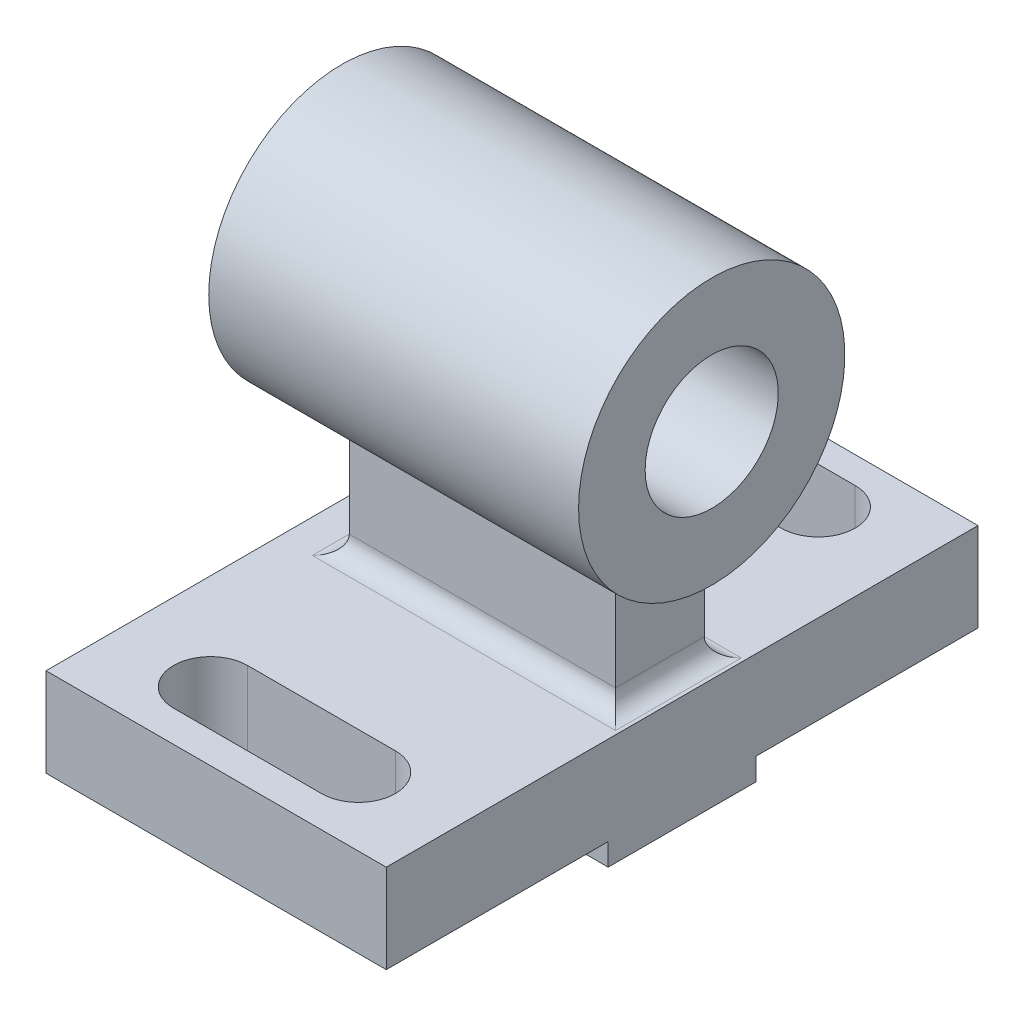
ISO-10303-21;
HEADER;
FILE_DESCRIPTION(('STEP AP214'),'2;1');
FILE_NAME('part.step','',(''),(''),'','','');
FILE_SCHEMA(('AUTOMOTIVE_DESIGN { 1 0 10303 214 1 1 1 1 }'));
ENDSEC;
DATA;
#1=APPLICATION_CONTEXT('core data for automotive mechanical design processes');
#2=APPLICATION_PROTOCOL_DEFINITION('international standard','automotive_design',2000,#1);
#3=PRODUCT_CONTEXT('',#1,'mechanical');
#4=PRODUCT('Part','Part','',(#3));
#5=PRODUCT_RELATED_PRODUCT_CATEGORY('part','',(#4));
#6=PRODUCT_DEFINITION_FORMATION('','',#4);
#7=PRODUCT_DEFINITION_CONTEXT('part definition',#1,'design');
#8=PRODUCT_DEFINITION('design','',#6,#7);
#9=PRODUCT_DEFINITION_SHAPE('','',#8);
#10=(LENGTH_UNIT() NAMED_UNIT(*) SI_UNIT(.MILLI.,.METRE.));
#11=(NAMED_UNIT(*) PLANE_ANGLE_UNIT() SI_UNIT($,.RADIAN.));
#12=(NAMED_UNIT(*) SI_UNIT($,.STERADIAN.) SOLID_ANGLE_UNIT());
#13=UNCERTAINTY_MEASURE_WITH_UNIT(LENGTH_MEASURE(1.E-05),#10,'distance_accuracy_value','');
#14=(GEOMETRIC_REPRESENTATION_CONTEXT(3) GLOBAL_UNCERTAINTY_ASSIGNED_CONTEXT((#13)) GLOBAL_UNIT_ASSIGNED_CONTEXT((#10,
#11,#12)) REPRESENTATION_CONTEXT('',''));
#15=CARTESIAN_POINT('',(0.,0.,0.));
#16=DIRECTION('',(0.,0.,1.));
#17=DIRECTION('',(1.,0.,0.));
#18=AXIS2_PLACEMENT_3D('',#15,#16,#17);
#19=CARTESIAN_POINT('',(46.,12.,-80.));
#20=DIRECTION('',(0.,-1.,0.));
#21=DIRECTION('',(0.,0.,-1.));
#22=AXIS2_PLACEMENT_3D('',#19,#20,#21);
#23=PLANE('',#22);
#24=DIRECTION('',(0.,0.,-1.));
#25=VECTOR('',#24,1.);
#26=CARTESIAN_POINT('',(4.50000000000001,12.,-80.));
#27=LINE('',#26,#25);
#28=CARTESIAN_POINT('',(4.50000000000001,12.,-31.5));
#29=VERTEX_POINT('',#28);
#30=CARTESIAN_POINT('',(4.50000000000001,12.,-48.5));
#31=VERTEX_POINT('',#30);
#32=EDGE_CURVE('E364',#29,#31,#27,.T.);
#33=ORIENTED_EDGE('',*,*,#32,.T.);
#34=DIRECTION('',(-1.,0.,0.));
#35=VECTOR('',#34,1.);
#36=CARTESIAN_POINT('',(43.,12.,-48.5));
#37=LINE('',#36,#35);
#38=CARTESIAN_POINT('',(45.5,12.,-48.5));
#39=VERTEX_POINT('',#38);
#40=EDGE_CURVE('E366',#31,#39,#37,.F.);
#41=ORIENTED_EDGE('',*,*,#40,.T.);
#42=DIRECTION('',(0.,0.,-1.));
#43=VECTOR('',#42,1.);
#44=CARTESIAN_POINT('',(45.5,12.,-34.));
#45=LINE('',#44,#43);
#46=CARTESIAN_POINT('',(45.5,12.,-31.5));
#47=VERTEX_POINT('',#46);
#48=EDGE_CURVE('E365',#39,#47,#45,.F.);
#49=ORIENTED_EDGE('',*,*,#48,.T.);
#50=DIRECTION('',(-1.,0.,0.));
#51=VECTOR('',#50,1.);
#52=CARTESIAN_POINT('',(46.,12.,-31.5));
#53=LINE('',#52,#51);
#54=EDGE_CURVE('E359',#47,#29,#53,.T.);
#55=ORIENTED_EDGE('',*,*,#54,.T.);
#56=EDGE_LOOP('',(#33,#41,#49,#55));
#57=FACE_BOUND('',#56,.T.);
#58=DIRECTION('',(1.,0.,0.));
#59=VECTOR('',#58,1.);
#60=CARTESIAN_POINT('',(13.,12.,-66.3852254242808));
#61=LINE('',#60,#59);
#62=CARTESIAN_POINT('',(13.,12.,-66.3852254242808));
#63=VERTEX_POINT('',#62);
#64=CARTESIAN_POINT('',(33.,12.,-66.3852254242808));
#65=VERTEX_POINT('',#64);
#66=EDGE_CURVE('E209',#63,#65,#61,.T.);
#67=ORIENTED_EDGE('',*,*,#66,.F.);
#68=CARTESIAN_POINT('',(13.,12.,-71.3852254242809));
#69=DIRECTION('',(0.,1.,0.));
#70=DIRECTION('',(0.,0.,1.));
#71=AXIS2_PLACEMENT_3D('',#68,#69,#70);
#72=CIRCLE('',#71,5.);
#73=CARTESIAN_POINT('',(13.,12.,-76.3852254242809));
#74=VERTEX_POINT('',#73);
#75=EDGE_CURVE('E211',#74,#63,#72,.T.);
#76=ORIENTED_EDGE('',*,*,#75,.F.);
#77=DIRECTION('',(-1.,0.,0.));
#78=VECTOR('',#77,1.);
#79=CARTESIAN_POINT('',(13.,12.,-76.3852254242809));
#80=LINE('',#79,#78);
#81=CARTESIAN_POINT('',(33.,12.,-76.3852254242809));
#82=VERTEX_POINT('',#81);
#83=EDGE_CURVE('E219',#82,#74,#80,.T.);
#84=ORIENTED_EDGE('',*,*,#83,.F.);
#85=CARTESIAN_POINT('',(33.,12.,-71.3852254242809));
#86=DIRECTION('',(0.,1.,0.));
#87=DIRECTION('',(0.,0.,1.));
#88=AXIS2_PLACEMENT_3D('',#85,#86,#87);
#89=CIRCLE('',#88,5.);
#90=EDGE_CURVE('E199',#65,#82,#89,.T.);
#91=ORIENTED_EDGE('',*,*,#90,.F.);
#92=EDGE_LOOP('',(#67,#76,#84,#91));
#93=FACE_BOUND('',#92,.T.);
#94=DIRECTION('',(1.,0.,0.));
#95=VECTOR('',#94,1.);
#96=CARTESIAN_POINT('',(13.,12.,-4.2432780191033));
#97=LINE('',#96,#95);
#98=CARTESIAN_POINT('',(13.,12.,-4.24327801910331));
#99=VERTEX_POINT('',#98);
#100=CARTESIAN_POINT('',(33.,12.,-4.2432780191033));
#101=VERTEX_POINT('',#100);
#102=EDGE_CURVE('E243',#99,#101,#97,.T.);
#103=ORIENTED_EDGE('',*,*,#102,.F.);
#104=CARTESIAN_POINT('',(13.,12.,-9.2432780191033));
#105=DIRECTION('',(0.,1.,0.));
#106=DIRECTION('',(0.,0.,1.));
#107=AXIS2_PLACEMENT_3D('',#104,#105,#106);
#108=CIRCLE('',#107,5.);
#109=CARTESIAN_POINT('',(13.,12.,-14.2432780191033));
#110=VERTEX_POINT('',#109);
#111=EDGE_CURVE('E246',#110,#99,#108,.T.);
#112=ORIENTED_EDGE('',*,*,#111,.F.);
#113=DIRECTION('',(-1.,0.,0.));
#114=VECTOR('',#113,1.);
#115=CARTESIAN_POINT('',(13.,12.,-14.2432780191033));
#116=LINE('',#115,#114);
#117=CARTESIAN_POINT('',(33.,12.,-14.2432780191033));
#118=VERTEX_POINT('',#117);
#119=EDGE_CURVE('E233',#118,#110,#116,.T.);
#120=ORIENTED_EDGE('',*,*,#119,.F.);
#121=CARTESIAN_POINT('',(33.,12.,-9.2432780191033));
#122=DIRECTION('',(0.,1.,0.));
#123=DIRECTION('',(0.,0.,1.));
#124=AXIS2_PLACEMENT_3D('',#121,#122,#123);
#125=CIRCLE('',#124,5.);
#126=EDGE_CURVE('E239',#101,#118,#125,.T.);
#127=ORIENTED_EDGE('',*,*,#126,.F.);
#128=EDGE_LOOP('',(#103,#112,#120,#127));
#129=FACE_BOUND('',#128,.T.);
#130=DIRECTION('',(0.,0.,1.));
#131=VECTOR('',#130,1.);
#132=CARTESIAN_POINT('',(0.,12.,-80.));
#133=LINE('',#132,#131);
#134=CARTESIAN_POINT('',(0.,12.,-80.));
#135=VERTEX_POINT('',#134);
#136=CARTESIAN_POINT('',(0.,12.,0.));
#137=VERTEX_POINT('',#136);
#138=EDGE_CURVE('E297',#135,#137,#133,.T.);
#139=ORIENTED_EDGE('',*,*,#138,.T.);
#140=DIRECTION('',(-1.,0.,0.));
#141=VECTOR('',#140,1.);
#142=CARTESIAN_POINT('',(46.,12.,0.));
#143=LINE('',#142,#141);
#144=CARTESIAN_POINT('',(46.,12.,0.));
#145=VERTEX_POINT('',#144);
#146=EDGE_CURVE('E328',#145,#137,#143,.T.);
#147=ORIENTED_EDGE('',*,*,#146,.F.);
#148=DIRECTION('',(0.,0.,1.));
#149=VECTOR('',#148,1.);
#150=CARTESIAN_POINT('',(46.,12.,-80.));
#151=LINE('',#150,#149);
#152=CARTESIAN_POINT('',(46.,12.,-80.));
#153=VERTEX_POINT('',#152);
#154=EDGE_CURVE('E285',#153,#145,#151,.T.);
#155=ORIENTED_EDGE('',*,*,#154,.F.);
#156=DIRECTION('',(-1.,0.,0.));
#157=VECTOR('',#156,1.);
#158=CARTESIAN_POINT('',(46.,12.,-80.));
#159=LINE('',#158,#157);
#160=EDGE_CURVE('E334',#153,#135,#159,.T.);
#161=ORIENTED_EDGE('',*,*,#160,.T.);
#162=EDGE_LOOP('',(#139,#147,#155,#161));
#163=FACE_BOUND('',#162,.T.);
#164=ADVANCED_FACE('F41',(#57,#93,#129,#163),#23,.F.);
#165=CARTESIAN_POINT('',(46.,0.,-80.));
#166=DIRECTION('',(0.,0.,1.));
#167=DIRECTION('',(1.,0.,0.));
#168=AXIS2_PLACEMENT_3D('',#165,#166,#167);
#169=PLANE('',#168);
#170=DIRECTION('',(0.,1.,0.));
#171=VECTOR('',#170,1.);
#172=CARTESIAN_POINT('',(0.,0.,-80.));
#173=LINE('',#172,#171);
#174=CARTESIAN_POINT('',(0.,0.,-80.));
#175=VERTEX_POINT('',#174);
#176=EDGE_CURVE('E279',#175,#135,#173,.T.);
#177=ORIENTED_EDGE('',*,*,#176,.T.);
#178=ORIENTED_EDGE('',*,*,#160,.F.);
#179=DIRECTION('',(0.,1.,0.));
#180=VECTOR('',#179,1.);
#181=CARTESIAN_POINT('',(46.,0.,-80.));
#182=LINE('',#181,#180);
#183=CARTESIAN_POINT('',(46.,0.,-80.));
#184=VERTEX_POINT('',#183);
#185=EDGE_CURVE('E276',#184,#153,#182,.T.);
#186=ORIENTED_EDGE('',*,*,#185,.F.);
#187=DIRECTION('',(-1.,0.,0.));
#188=VECTOR('',#187,1.);
#189=CARTESIAN_POINT('',(46.,0.,-80.));
#190=LINE('',#189,#188);
#191=EDGE_CURVE('E300',#184,#175,#190,.T.);
#192=ORIENTED_EDGE('',*,*,#191,.T.);
#193=EDGE_LOOP('',(#177,#178,#186,#192));
#194=FACE_BOUND('',#193,.T.);
#195=ADVANCED_FACE('F423',(#194),#169,.F.);
#196=CARTESIAN_POINT('',(46.,12.,0.));
#197=DIRECTION('',(0.,0.,-1.));
#198=DIRECTION('',(-1.,0.,0.));
#199=AXIS2_PLACEMENT_3D('',#196,#197,#198);
#200=PLANE('',#199);
#201=DIRECTION('',(0.,-1.,0.));
#202=VECTOR('',#201,1.);
#203=CARTESIAN_POINT('',(0.,12.,0.));
#204=LINE('',#203,#202);
#205=CARTESIAN_POINT('',(0.,0.,0.));
#206=VERTEX_POINT('',#205);
#207=EDGE_CURVE('E305',#137,#206,#204,.T.);
#208=ORIENTED_EDGE('',*,*,#207,.T.);
#209=DIRECTION('',(-1.,0.,0.));
#210=VECTOR('',#209,1.);
#211=CARTESIAN_POINT('',(46.,0.,0.));
#212=LINE('',#211,#210);
#213=CARTESIAN_POINT('',(46.,0.,0.));
#214=VERTEX_POINT('',#213);
#215=EDGE_CURVE('E330',#214,#206,#212,.T.);
#216=ORIENTED_EDGE('',*,*,#215,.F.);
#217=DIRECTION('',(0.,-1.,0.));
#218=VECTOR('',#217,1.);
#219=CARTESIAN_POINT('',(46.,12.,0.));
#220=LINE('',#219,#218);
#221=EDGE_CURVE('E283',#145,#214,#220,.T.);
#222=ORIENTED_EDGE('',*,*,#221,.F.);
#223=ORIENTED_EDGE('',*,*,#146,.T.);
#224=EDGE_LOOP('',(#208,#216,#222,#223));
#225=FACE_BOUND('',#224,.T.);
#226=ADVANCED_FACE('F430',(#225),#200,.F.);
#227=CARTESIAN_POINT('',(46.,0.,0.));
#228=DIRECTION('',(0.,1.,0.));
#229=DIRECTION('',(0.,0.,1.));
#230=AXIS2_PLACEMENT_3D('',#227,#228,#229);
#231=PLANE('',#230);
#232=DIRECTION('',(-1.,0.,0.));
#233=VECTOR('',#232,1.);
#234=CARTESIAN_POINT('',(46.,0.,-14.2432780191033));
#235=LINE('',#234,#233);
#236=CARTESIAN_POINT('',(33.,0.,-14.2432780191033));
#237=VERTEX_POINT('',#236);
#238=CARTESIAN_POINT('',(13.,0.,-14.2432780191033));
#239=VERTEX_POINT('',#238);
#240=EDGE_CURVE('E351',#237,#239,#235,.T.);
#241=ORIENTED_EDGE('',*,*,#240,.T.);
#242=CARTESIAN_POINT('',(13.,0.,-9.2432780191033));
#243=DIRECTION('',(0.,1.,0.));
#244=DIRECTION('',(0.,0.,1.));
#245=AXIS2_PLACEMENT_3D('',#242,#243,#244);
#246=CIRCLE('',#245,5.);
#247=CARTESIAN_POINT('',(13.,0.,-4.2432780191033));
#248=VERTEX_POINT('',#247);
#249=EDGE_CURVE('E353',#239,#248,#246,.T.);
#250=ORIENTED_EDGE('',*,*,#249,.T.);
#251=DIRECTION('',(1.,0.,0.));
#252=VECTOR('',#251,1.);
#253=CARTESIAN_POINT('',(46.,0.,-4.2432780191033));
#254=LINE('',#253,#252);
#255=CARTESIAN_POINT('',(33.,0.,-4.2432780191033));
#256=VERTEX_POINT('',#255);
#257=EDGE_CURVE('E343',#248,#256,#254,.T.);
#258=ORIENTED_EDGE('',*,*,#257,.T.);
#259=CARTESIAN_POINT('',(33.,0.,-9.2432780191033));
#260=DIRECTION('',(0.,1.,0.));
#261=DIRECTION('',(0.,0.,1.));
#262=AXIS2_PLACEMENT_3D('',#259,#260,#261);
#263=CIRCLE('',#262,5.);
#264=EDGE_CURVE('E349',#256,#237,#263,.T.);
#265=ORIENTED_EDGE('',*,*,#264,.T.);
#266=EDGE_LOOP('',(#241,#250,#258,#265));
#267=FACE_BOUND('',#266,.T.);
#268=DIRECTION('',(0.,0.,-1.));
#269=VECTOR('',#268,1.);
#270=CARTESIAN_POINT('',(0.,0.,0.));
#271=LINE('',#270,#269);
#272=CARTESIAN_POINT('',(0.,0.,-30.));
#273=VERTEX_POINT('',#272);
#274=EDGE_CURVE('E302',#206,#273,#271,.T.);
#275=ORIENTED_EDGE('',*,*,#274,.T.);
#276=DIRECTION('',(-1.,0.,0.));
#277=VECTOR('',#276,1.);
#278=CARTESIAN_POINT('',(46.,0.,-30.));
#279=LINE('',#278,#277);
#280=CARTESIAN_POINT('',(46.,0.,-30.));
#281=VERTEX_POINT('',#280);
#282=EDGE_CURVE('E321',#281,#273,#279,.T.);
#283=ORIENTED_EDGE('',*,*,#282,.F.);
#284=DIRECTION('',(0.,0.,-1.));
#285=VECTOR('',#284,1.);
#286=CARTESIAN_POINT('',(46.,0.,0.));
#287=LINE('',#286,#285);
#288=EDGE_CURVE('E287',#214,#281,#287,.T.);
#289=ORIENTED_EDGE('',*,*,#288,.F.);
#290=ORIENTED_EDGE('',*,*,#215,.T.);
#291=EDGE_LOOP('',(#275,#283,#289,#290));
#292=FACE_BOUND('',#291,.T.);
#293=ADVANCED_FACE('F498',(#267,#292),#231,.F.);
#294=CARTESIAN_POINT('',(46.,0.,-30.));
#295=DIRECTION('',(0.,0.,-1.));
#296=DIRECTION('',(-1.,0.,0.));
#297=AXIS2_PLACEMENT_3D('',#294,#295,#296);
#298=PLANE('',#297);
#299=DIRECTION('',(0.,-1.,0.));
#300=VECTOR('',#299,1.);
#301=CARTESIAN_POINT('',(0.,0.,-30.));
#302=LINE('',#301,#300);
#303=CARTESIAN_POINT('',(0.,-3.,-30.));
#304=VERTEX_POINT('',#303);
#305=EDGE_CURVE('E306',#273,#304,#302,.T.);
#306=ORIENTED_EDGE('',*,*,#305,.T.);
#307=DIRECTION('',(-1.,0.,0.));
#308=VECTOR('',#307,1.);
#309=CARTESIAN_POINT('',(46.,-3.,-30.));
#310=LINE('',#309,#308);
#311=CARTESIAN_POINT('',(46.,-3.,-30.));
#312=VERTEX_POINT('',#311);
#313=EDGE_CURVE('E322',#312,#304,#310,.T.);
#314=ORIENTED_EDGE('',*,*,#313,.F.);
#315=DIRECTION('',(0.,-1.,0.));
#316=VECTOR('',#315,1.);
#317=CARTESIAN_POINT('',(46.,0.,-30.));
#318=LINE('',#317,#316);
#319=EDGE_CURVE('E288',#281,#312,#318,.T.);
#320=ORIENTED_EDGE('',*,*,#319,.F.);
#321=ORIENTED_EDGE('',*,*,#282,.T.);
#322=EDGE_LOOP('',(#306,#314,#320,#321));
#323=FACE_BOUND('',#322,.T.);
#324=ADVANCED_FACE('F492',(#323),#298,.F.);
#325=CARTESIAN_POINT('',(46.,-3.,-30.));
#326=DIRECTION('',(0.,1.,0.));
#327=DIRECTION('',(0.,0.,1.));
#328=AXIS2_PLACEMENT_3D('',#325,#326,#327);
#329=PLANE('',#328);
#330=DIRECTION('',(0.,0.,-1.));
#331=VECTOR('',#330,1.);
#332=CARTESIAN_POINT('',(0.,-3.,-30.));
#333=LINE('',#332,#331);
#334=CARTESIAN_POINT('',(0.,-3.,-50.));
#335=VERTEX_POINT('',#334);
#336=EDGE_CURVE('E308',#304,#335,#333,.T.);
#337=ORIENTED_EDGE('',*,*,#336,.T.);
#338=DIRECTION('',(-1.,0.,0.));
#339=VECTOR('',#338,1.);
#340=CARTESIAN_POINT('',(46.,-3.,-50.));
#341=LINE('',#340,#339);
#342=CARTESIAN_POINT('',(46.,-3.,-50.));
#343=VERTEX_POINT('',#342);
#344=EDGE_CURVE('E319',#343,#335,#341,.T.);
#345=ORIENTED_EDGE('',*,*,#344,.F.);
#346=DIRECTION('',(0.,0.,-1.));
#347=VECTOR('',#346,1.);
#348=CARTESIAN_POINT('',(46.,-3.,-30.));
#349=LINE('',#348,#347);
#350=EDGE_CURVE('E293',#312,#343,#349,.T.);
#351=ORIENTED_EDGE('',*,*,#350,.F.);
#352=ORIENTED_EDGE('',*,*,#313,.T.);
#353=EDGE_LOOP('',(#337,#345,#351,#352));
#354=FACE_BOUND('',#353,.T.);
#355=ADVANCED_FACE('F493',(#354),#329,.F.);
#356=CARTESIAN_POINT('',(46.,-3.,-50.));
#357=DIRECTION('',(0.,0.,1.));
#358=DIRECTION('',(1.,0.,0.));
#359=AXIS2_PLACEMENT_3D('',#356,#357,#358);
#360=PLANE('',#359);
#361=DIRECTION('',(0.,1.,0.));
#362=VECTOR('',#361,1.);
#363=CARTESIAN_POINT('',(0.,-3.,-50.));
#364=LINE('',#363,#362);
#365=CARTESIAN_POINT('',(0.,0.,-50.));
#366=VERTEX_POINT('',#365);
#367=EDGE_CURVE('E309',#335,#366,#364,.T.);
#368=ORIENTED_EDGE('',*,*,#367,.T.);
#369=DIRECTION('',(-1.,0.,0.));
#370=VECTOR('',#369,1.);
#371=CARTESIAN_POINT('',(46.,0.,-50.));
#372=LINE('',#371,#370);
#373=CARTESIAN_POINT('',(46.,0.,-50.));
#374=VERTEX_POINT('',#373);
#375=EDGE_CURVE('E314',#374,#366,#372,.T.);
#376=ORIENTED_EDGE('',*,*,#375,.F.);
#377=DIRECTION('',(0.,1.,0.));
#378=VECTOR('',#377,1.);
#379=CARTESIAN_POINT('',(46.,-3.,-50.));
#380=LINE('',#379,#378);
#381=EDGE_CURVE('E291',#343,#374,#380,.T.);
#382=ORIENTED_EDGE('',*,*,#381,.F.);
#383=ORIENTED_EDGE('',*,*,#344,.T.);
#384=EDGE_LOOP('',(#368,#376,#382,#383));
#385=FACE_BOUND('',#384,.T.);
#386=ADVANCED_FACE('F487',(#385),#360,.F.);
#387=CARTESIAN_POINT('',(46.,0.,-50.));
#388=DIRECTION('',(0.,1.,0.));
#389=DIRECTION('',(0.,0.,1.));
#390=AXIS2_PLACEMENT_3D('',#387,#388,#389);
#391=PLANE('',#390);
#392=DIRECTION('',(-1.,0.,0.));
#393=VECTOR('',#392,1.);
#394=CARTESIAN_POINT('',(46.,0.,-76.3852254242809));
#395=LINE('',#394,#393);
#396=CARTESIAN_POINT('',(33.,0.,-76.3852254242809));
#397=VERTEX_POINT('',#396);
#398=CARTESIAN_POINT('',(13.,0.,-76.3852254242809));
#399=VERTEX_POINT('',#398);
#400=EDGE_CURVE('E339',#397,#399,#395,.T.);
#401=ORIENTED_EDGE('',*,*,#400,.T.);
#402=CARTESIAN_POINT('',(13.,0.,-71.3852254242809));
#403=DIRECTION('',(0.,1.,0.));
#404=DIRECTION('',(0.,0.,1.));
#405=AXIS2_PLACEMENT_3D('',#402,#403,#404);
#406=CIRCLE('',#405,5.);
#407=CARTESIAN_POINT('',(13.,0.,-66.3852254242808));
#408=VERTEX_POINT('',#407);
#409=EDGE_CURVE('E345',#399,#408,#406,.T.);
#410=ORIENTED_EDGE('',*,*,#409,.T.);
#411=DIRECTION('',(1.,0.,0.));
#412=VECTOR('',#411,1.);
#413=CARTESIAN_POINT('',(46.,0.,-66.3852254242808));
#414=LINE('',#413,#412);
#415=CARTESIAN_POINT('',(33.,0.,-66.3852254242808));
#416=VERTEX_POINT('',#415);
#417=EDGE_CURVE('E337',#408,#416,#414,.T.);
#418=ORIENTED_EDGE('',*,*,#417,.T.);
#419=CARTESIAN_POINT('',(33.,0.,-71.3852254242809));
#420=DIRECTION('',(0.,1.,0.));
#421=DIRECTION('',(0.,0.,1.));
#422=AXIS2_PLACEMENT_3D('',#419,#420,#421);
#423=CIRCLE('',#422,5.);
#424=EDGE_CURVE('E201',#416,#397,#423,.T.);
#425=ORIENTED_EDGE('',*,*,#424,.T.);
#426=EDGE_LOOP('',(#401,#410,#418,#425));
#427=FACE_BOUND('',#426,.T.);
#428=DIRECTION('',(0.,0.,-1.));
#429=VECTOR('',#428,1.);
#430=CARTESIAN_POINT('',(0.,0.,-50.));
#431=LINE('',#430,#429);
#432=EDGE_CURVE('E284',#366,#175,#431,.T.);
#433=ORIENTED_EDGE('',*,*,#432,.T.);
#434=ORIENTED_EDGE('',*,*,#191,.F.);
#435=DIRECTION('',(0.,0.,-1.));
#436=VECTOR('',#435,1.);
#437=CARTESIAN_POINT('',(46.,0.,-50.));
#438=LINE('',#437,#436);
#439=EDGE_CURVE('E294',#374,#184,#438,.T.);
#440=ORIENTED_EDGE('',*,*,#439,.F.);
#441=ORIENTED_EDGE('',*,*,#375,.T.);
#442=EDGE_LOOP('',(#433,#434,#440,#441));
#443=FACE_BOUND('',#442,.T.);
#444=ADVANCED_FACE('F482',(#427,#443),#391,.F.);
#445=CARTESIAN_POINT('',(46.,0.,0.));
#446=DIRECTION('',(1.,0.,0.));
#447=DIRECTION('',(0.,0.,-1.));
#448=AXIS2_PLACEMENT_3D('',#445,#446,#447);
#449=PLANE('',#448);
#450=ORIENTED_EDGE('',*,*,#185,.T.);
#451=ORIENTED_EDGE('',*,*,#154,.T.);
#452=ORIENTED_EDGE('',*,*,#221,.T.);
#453=ORIENTED_EDGE('',*,*,#288,.T.);
#454=ORIENTED_EDGE('',*,*,#319,.T.);
#455=ORIENTED_EDGE('',*,*,#350,.T.);
#456=ORIENTED_EDGE('',*,*,#381,.T.);
#457=ORIENTED_EDGE('',*,*,#439,.T.);
#458=EDGE_LOOP('',(#450,#451,#452,#453,#454,#455,#456,#457));
#459=FACE_BOUND('',#458,.T.);
#460=ADVANCED_FACE('F417',(#459),#449,.T.);
#461=CARTESIAN_POINT('',(0.,0.,0.));
#462=DIRECTION('',(1.,0.,0.));
#463=DIRECTION('',(0.,0.,-1.));
#464=AXIS2_PLACEMENT_3D('',#461,#462,#463);
#465=PLANE('',#464);
#466=ORIENTED_EDGE('',*,*,#176,.F.);
#467=ORIENTED_EDGE('',*,*,#432,.F.);
#468=ORIENTED_EDGE('',*,*,#367,.F.);
#469=ORIENTED_EDGE('',*,*,#336,.F.);
#470=ORIENTED_EDGE('',*,*,#305,.F.);
#471=ORIENTED_EDGE('',*,*,#274,.F.);
#472=ORIENTED_EDGE('',*,*,#207,.F.);
#473=ORIENTED_EDGE('',*,*,#138,.F.);
#474=EDGE_LOOP('',(#466,#467,#468,#469,#470,#471,#472,#473));
#475=FACE_BOUND('',#474,.T.);
#476=ADVANCED_FACE('F406',(#475),#465,.F.);
#477=CARTESIAN_POINT('',(43.,63.001,-34.));
#478=DIRECTION('',(0.,0.,1.));
#479=DIRECTION('',(1.,0.,0.));
#480=AXIS2_PLACEMENT_3D('',#477,#478,#479);
#481=PLANE('',#480);
#482=DIRECTION('',(0.,-1.,0.));
#483=VECTOR('',#482,1.);
#484=CARTESIAN_POINT('',(7.00000000000001,63.001,-34.));
#485=LINE('',#484,#483);
#486=CARTESIAN_POINT('',(7.00000000000001,28.0294372515229,-34.));
#487=VERTEX_POINT('',#486);
#488=CARTESIAN_POINT('',(7.00000000000001,14.5,-34.));
#489=VERTEX_POINT('',#488);
#490=EDGE_CURVE('E272',#487,#489,#485,.T.);
#491=ORIENTED_EDGE('',*,*,#490,.T.);
#492=DIRECTION('',(-1.,0.,0.));
#493=VECTOR('',#492,1.);
#494=CARTESIAN_POINT('',(43.,14.5,-34.));
#495=LINE('',#494,#493);
#496=CARTESIAN_POINT('',(43.,14.5,-34.));
#497=VERTEX_POINT('',#496);
#498=EDGE_CURVE('E11',#489,#497,#495,.F.);
#499=ORIENTED_EDGE('',*,*,#498,.T.);
#500=DIRECTION('',(0.,-1.,0.));
#501=VECTOR('',#500,1.);
#502=CARTESIAN_POINT('',(43.,63.001,-34.));
#503=LINE('',#502,#501);
#504=CARTESIAN_POINT('',(43.,28.0294372515229,-34.));
#505=VERTEX_POINT('',#504);
#506=EDGE_CURVE('E260',#505,#497,#503,.T.);
#507=ORIENTED_EDGE('',*,*,#506,.F.);
#508=DIRECTION('',(-1.,0.,0.));
#509=VECTOR('',#508,1.);
#510=CARTESIAN_POINT('',(50.,28.0294372515229,-34.));
#511=LINE('',#510,#509);
#512=EDGE_CURVE('E268',#487,#505,#511,.F.);
#513=ORIENTED_EDGE('',*,*,#512,.F.);
#514=EDGE_LOOP('',(#491,#499,#507,#513));
#515=FACE_BOUND('',#514,.T.);
#516=ADVANCED_FACE('F410',(#515),#481,.T.);
#517=CARTESIAN_POINT('',(7.00000000000001,63.001,-34.));
#518=DIRECTION('',(-1.,0.,0.));
#519=DIRECTION('',(0.,0.,1.));
#520=AXIS2_PLACEMENT_3D('',#517,#518,#519);
#521=PLANE('',#520);
#522=DIRECTION('',(0.,-1.,0.));
#523=VECTOR('',#522,1.);
#524=CARTESIAN_POINT('',(7.00000000000001,63.001,-46.));
#525=LINE('',#524,#523);
#526=CARTESIAN_POINT('',(7.00000000000001,28.0294372515229,-46.));
#527=VERTEX_POINT('',#526);
#528=CARTESIAN_POINT('',(7.00000000000001,14.5,-46.));
#529=VERTEX_POINT('',#528);
#530=EDGE_CURVE('E271',#527,#529,#525,.T.);
#531=ORIENTED_EDGE('',*,*,#530,.T.);
#532=DIRECTION('',(0.,0.,-1.));
#533=VECTOR('',#532,1.);
#534=CARTESIAN_POINT('',(7.00000000000001,14.5,-34.));
#535=LINE('',#534,#533);
#536=EDGE_CURVE('E61',#529,#489,#535,.F.);
#537=ORIENTED_EDGE('',*,*,#536,.T.);
#538=ORIENTED_EDGE('',*,*,#490,.F.);
#539=CARTESIAN_POINT('',(7.00000000000001,45.,-40.));
#540=DIRECTION('',(-1.,0.,0.));
#541=DIRECTION('',(0.,0.,1.));
#542=AXIS2_PLACEMENT_3D('',#539,#540,#541);
#543=CIRCLE('',#542,18.);
#544=EDGE_CURVE('E258',#527,#487,#543,.T.);
#545=ORIENTED_EDGE('',*,*,#544,.F.);
#546=EDGE_LOOP('',(#531,#537,#538,#545));
#547=FACE_BOUND('',#546,.T.);
#548=ADVANCED_FACE('F400',(#547),#521,.T.);
#549=CARTESIAN_POINT('',(43.,63.001,-46.));
#550=DIRECTION('',(0.,0.,1.));
#551=DIRECTION('',(1.,0.,0.));
#552=AXIS2_PLACEMENT_3D('',#549,#550,#551);
#553=PLANE('',#552);
#554=DIRECTION('',(0.,-1.,0.));
#555=VECTOR('',#554,1.);
#556=CARTESIAN_POINT('',(43.,63.001,-46.));
#557=LINE('',#556,#555);
#558=CARTESIAN_POINT('',(43.,28.0294372515229,-46.));
#559=VERTEX_POINT('',#558);
#560=CARTESIAN_POINT('',(43.,14.5,-46.));
#561=VERTEX_POINT('',#560);
#562=EDGE_CURVE('E264',#559,#561,#557,.T.);
#563=ORIENTED_EDGE('',*,*,#562,.T.);
#564=DIRECTION('',(-1.,0.,0.));
#565=VECTOR('',#564,1.);
#566=CARTESIAN_POINT('',(7.00000000000001,14.5,-46.));
#567=LINE('',#566,#565);
#568=EDGE_CURVE('E357',#561,#529,#567,.T.);
#569=ORIENTED_EDGE('',*,*,#568,.T.);
#570=ORIENTED_EDGE('',*,*,#530,.F.);
#571=DIRECTION('',(-1.,0.,0.));
#572=VECTOR('',#571,1.);
#573=CARTESIAN_POINT('',(50.,28.0294372515229,-46.));
#574=LINE('',#573,#572);
#575=EDGE_CURVE('E265',#527,#559,#574,.F.);
#576=ORIENTED_EDGE('',*,*,#575,.T.);
#577=EDGE_LOOP('',(#563,#569,#570,#576));
#578=FACE_BOUND('',#577,.T.);
#579=ADVANCED_FACE('F397',(#578),#553,.F.);
#580=CARTESIAN_POINT('',(43.,63.001,-34.));
#581=DIRECTION('',(-1.,0.,0.));
#582=DIRECTION('',(0.,0.,1.));
#583=AXIS2_PLACEMENT_3D('',#580,#581,#582);
#584=PLANE('',#583);
#585=ORIENTED_EDGE('',*,*,#506,.T.);
#586=DIRECTION('',(0.,0.,-1.));
#587=VECTOR('',#586,1.);
#588=CARTESIAN_POINT('',(43.,14.5,-46.));
#589=LINE('',#588,#587);
#590=EDGE_CURVE('E49',#497,#561,#589,.T.);
#591=ORIENTED_EDGE('',*,*,#590,.T.);
#592=ORIENTED_EDGE('',*,*,#562,.F.);
#593=CARTESIAN_POINT('',(43.,45.,-40.));
#594=DIRECTION('',(-1.,0.,0.));
#595=DIRECTION('',(0.,0.,1.));
#596=AXIS2_PLACEMENT_3D('',#593,#594,#595);
#597=CIRCLE('',#596,18.);
#598=EDGE_CURVE('E266',#559,#505,#597,.T.);
#599=ORIENTED_EDGE('',*,*,#598,.T.);
#600=EDGE_LOOP('',(#585,#591,#592,#599));
#601=FACE_BOUND('',#600,.T.);
#602=ADVANCED_FACE('F407',(#601),#584,.F.);
#603=CARTESIAN_POINT('',(50.,45.,-40.));
#604=DIRECTION('',(-1.,0.,0.));
#605=DIRECTION('',(0.,0.,1.));
#606=AXIS2_PLACEMENT_3D('',#603,#604,#605);
#607=CYLINDRICAL_SURFACE('',#606,18.);
#608=ORIENTED_EDGE('',*,*,#544,.T.);
#609=ORIENTED_EDGE('',*,*,#512,.T.);
#610=ORIENTED_EDGE('',*,*,#598,.F.);
#611=ORIENTED_EDGE('',*,*,#575,.F.);
#612=EDGE_LOOP('',(#608,#609,#610,#611));
#613=FACE_BOUND('',#612,.T.);
#614=CARTESIAN_POINT('',(50.,45.,-40.));
#615=DIRECTION('',(-1.,0.,0.));
#616=DIRECTION('',(0.,0.,1.));
#617=AXIS2_PLACEMENT_3D('',#614,#615,#616);
#618=CIRCLE('',#617,18.);
#619=CARTESIAN_POINT('',(50.,45.,-22.));
#620=VERTEX_POINT('',#619);
#621=EDGE_CURVE('E251',#620,#620,#618,.T.);
#622=ORIENTED_EDGE('',*,*,#621,.T.);
#623=EDGE_LOOP('',(#622));
#624=FACE_BOUND('',#623,.T.);
#625=CARTESIAN_POINT('',(0.,45.,-40.));
#626=DIRECTION('',(-1.,0.,0.));
#627=DIRECTION('',(0.,0.,1.));
#628=AXIS2_PLACEMENT_3D('',#625,#626,#627);
#629=CIRCLE('',#628,18.);
#630=CARTESIAN_POINT('',(0.,45.,-22.));
#631=VERTEX_POINT('',#630);
#632=EDGE_CURVE('E252',#631,#631,#629,.T.);
#633=ORIENTED_EDGE('',*,*,#632,.F.);
#634=EDGE_LOOP('',(#633));
#635=FACE_BOUND('',#634,.T.);
#636=ADVANCED_FACE('F401',(#613,#624,#635),#607,.T.);
#637=CARTESIAN_POINT('',(50.,45.,-40.));
#638=DIRECTION('',(-1.,0.,0.));
#639=DIRECTION('',(0.,0.,1.));
#640=AXIS2_PLACEMENT_3D('',#637,#638,#639);
#641=PLANE('',#640);
#642=CARTESIAN_POINT('',(50.,45.,-40.));
#643=DIRECTION('',(-1.,0.,0.));
#644=DIRECTION('',(0.,0.,1.));
#645=AXIS2_PLACEMENT_3D('',#642,#643,#644);
#646=CIRCLE('',#645,9.);
#647=CARTESIAN_POINT('',(50.,45.,-31.));
#648=VERTEX_POINT('',#647);
#649=EDGE_CURVE('E247',#648,#648,#646,.T.);
#650=ORIENTED_EDGE('',*,*,#649,.T.);
#651=EDGE_LOOP('',(#650));
#652=FACE_BOUND('',#651,.T.);
#653=ORIENTED_EDGE('',*,*,#621,.F.);
#654=EDGE_LOOP('',(#653));
#655=FACE_BOUND('',#654,.T.);
#656=ADVANCED_FACE('F467',(#652,#655),#641,.F.);
#657=CARTESIAN_POINT('',(0.,45.,-40.));
#658=DIRECTION('',(-1.,0.,0.));
#659=DIRECTION('',(0.,0.,1.));
#660=AXIS2_PLACEMENT_3D('',#657,#658,#659);
#661=PLANE('',#660);
#662=CARTESIAN_POINT('',(0.,45.,-40.));
#663=DIRECTION('',(-1.,0.,0.));
#664=DIRECTION('',(0.,0.,1.));
#665=AXIS2_PLACEMENT_3D('',#662,#663,#664);
#666=CIRCLE('',#665,9.);
#667=CARTESIAN_POINT('',(0.,45.,-31.));
#668=VERTEX_POINT('',#667);
#669=EDGE_CURVE('E225',#668,#668,#666,.T.);
#670=ORIENTED_EDGE('',*,*,#669,.F.);
#671=EDGE_LOOP('',(#670));
#672=FACE_BOUND('',#671,.T.);
#673=ORIENTED_EDGE('',*,*,#632,.T.);
#674=EDGE_LOOP('',(#673));
#675=FACE_BOUND('',#674,.T.);
#676=ADVANCED_FACE('F463',(#672,#675),#661,.T.);
#677=CARTESIAN_POINT('',(50.,45.,-40.));
#678=DIRECTION('',(-1.,0.,0.));
#679=DIRECTION('',(0.,0.,1.));
#680=AXIS2_PLACEMENT_3D('',#677,#678,#679);
#681=CYLINDRICAL_SURFACE('',#680,9.);
#682=ORIENTED_EDGE('',*,*,#649,.F.);
#683=EDGE_LOOP('',(#682));
#684=FACE_BOUND('',#683,.T.);
#685=ORIENTED_EDGE('',*,*,#669,.T.);
#686=EDGE_LOOP('',(#685));
#687=FACE_BOUND('',#686,.T.);
#688=ADVANCED_FACE('F458',(#684,#687),#681,.F.);
#689=CARTESIAN_POINT('',(13.,-3.,-71.3852254242809));
#690=DIRECTION('',(0.,1.,0.));
#691=DIRECTION('',(0.,0.,1.));
#692=AXIS2_PLACEMENT_3D('',#689,#690,#691);
#693=CYLINDRICAL_SURFACE('',#692,5.);
#694=DIRECTION('',(0.,1.,0.));
#695=VECTOR('',#694,1.);
#696=CARTESIAN_POINT('',(13.,-3.,-76.3852254242809));
#697=LINE('',#696,#695);
#698=EDGE_CURVE('E224',#399,#74,#697,.T.);
#699=ORIENTED_EDGE('',*,*,#698,.T.);
#700=ORIENTED_EDGE('',*,*,#75,.T.);
#701=DIRECTION('',(0.,1.,0.));
#702=VECTOR('',#701,1.);
#703=CARTESIAN_POINT('',(13.,-3.,-66.3852254242808));
#704=LINE('',#703,#702);
#705=EDGE_CURVE('E205',#408,#63,#704,.T.);
#706=ORIENTED_EDGE('',*,*,#705,.F.);
#707=ORIENTED_EDGE('',*,*,#409,.F.);
#708=EDGE_LOOP('',(#699,#700,#706,#707));
#709=FACE_BOUND('',#708,.T.);
#710=ADVANCED_FACE('F464',(#709),#693,.F.);
#711=CARTESIAN_POINT('',(13.,-3.,-76.3852254242809));
#712=DIRECTION('',(0.,0.,-1.));
#713=DIRECTION('',(0.,1.,0.));
#714=AXIS2_PLACEMENT_3D('',#711,#712,#713);
#715=PLANE('',#714);
#716=DIRECTION('',(0.,1.,0.));
#717=VECTOR('',#716,1.);
#718=CARTESIAN_POINT('',(33.,-3.,-76.3852254242809));
#719=LINE('',#718,#717);
#720=EDGE_CURVE('E203',#397,#82,#719,.T.);
#721=ORIENTED_EDGE('',*,*,#720,.T.);
#722=ORIENTED_EDGE('',*,*,#83,.T.);
#723=ORIENTED_EDGE('',*,*,#698,.F.);
#724=ORIENTED_EDGE('',*,*,#400,.F.);
#725=EDGE_LOOP('',(#721,#722,#723,#724));
#726=FACE_BOUND('',#725,.T.);
#727=ADVANCED_FACE('F549',(#726),#715,.F.);
#728=CARTESIAN_POINT('',(33.,-3.,-71.3852254242809));
#729=DIRECTION('',(0.,1.,0.));
#730=DIRECTION('',(0.,0.,1.));
#731=AXIS2_PLACEMENT_3D('',#728,#729,#730);
#732=CYLINDRICAL_SURFACE('',#731,5.);
#733=DIRECTION('',(0.,1.,0.));
#734=VECTOR('',#733,1.);
#735=CARTESIAN_POINT('',(33.,-3.,-66.3852254242808));
#736=LINE('',#735,#734);
#737=EDGE_CURVE('E194',#416,#65,#736,.T.);
#738=ORIENTED_EDGE('',*,*,#737,.T.);
#739=ORIENTED_EDGE('',*,*,#90,.T.);
#740=ORIENTED_EDGE('',*,*,#720,.F.);
#741=ORIENTED_EDGE('',*,*,#424,.F.);
#742=EDGE_LOOP('',(#738,#739,#740,#741));
#743=FACE_BOUND('',#742,.T.);
#744=ADVANCED_FACE('F193',(#743),#732,.F.);
#745=CARTESIAN_POINT('',(13.,-3.,-66.3852254242808));
#746=DIRECTION('',(0.,0.,1.));
#747=DIRECTION('',(0.,-1.,0.));
#748=AXIS2_PLACEMENT_3D('',#745,#746,#747);
#749=PLANE('',#748);
#750=ORIENTED_EDGE('',*,*,#705,.T.);
#751=ORIENTED_EDGE('',*,*,#66,.T.);
#752=ORIENTED_EDGE('',*,*,#737,.F.);
#753=ORIENTED_EDGE('',*,*,#417,.F.);
#754=EDGE_LOOP('',(#750,#751,#752,#753));
#755=FACE_BOUND('',#754,.T.);
#756=ADVANCED_FACE('F208',(#755),#749,.F.);
#757=CARTESIAN_POINT('',(13.,-3.00000000000001,-9.2432780191033));
#758=DIRECTION('',(0.,1.,0.));
#759=DIRECTION('',(0.,0.,1.));
#760=AXIS2_PLACEMENT_3D('',#757,#758,#759);
#761=CYLINDRICAL_SURFACE('',#760,5.);
#762=DIRECTION('',(0.,1.,0.));
#763=VECTOR('',#762,1.);
#764=CARTESIAN_POINT('',(13.,-3.00000000000001,-14.2432780191033));
#765=LINE('',#764,#763);
#766=EDGE_CURVE('E236',#239,#110,#765,.T.);
#767=ORIENTED_EDGE('',*,*,#766,.T.);
#768=ORIENTED_EDGE('',*,*,#111,.T.);
#769=DIRECTION('',(0.,1.,0.));
#770=VECTOR('',#769,1.);
#771=CARTESIAN_POINT('',(13.,-3.00000000000001,-4.2432780191033));
#772=LINE('',#771,#770);
#773=EDGE_CURVE('E226',#248,#99,#772,.T.);
#774=ORIENTED_EDGE('',*,*,#773,.F.);
#775=ORIENTED_EDGE('',*,*,#249,.F.);
#776=EDGE_LOOP('',(#767,#768,#774,#775));
#777=FACE_BOUND('',#776,.T.);
#778=ADVANCED_FACE('F451',(#777),#761,.F.);
#779=CARTESIAN_POINT('',(13.,-3.00000000000001,-14.2432780191033));
#780=DIRECTION('',(0.,0.,-1.));
#781=DIRECTION('',(0.,1.,0.));
#782=AXIS2_PLACEMENT_3D('',#779,#780,#781);
#783=PLANE('',#782);
#784=DIRECTION('',(0.,1.,0.));
#785=VECTOR('',#784,1.);
#786=CARTESIAN_POINT('',(33.,-3.00000000000001,-14.2432780191033));
#787=LINE('',#786,#785);
#788=EDGE_CURVE('E234',#237,#118,#787,.T.);
#789=ORIENTED_EDGE('',*,*,#788,.T.);
#790=ORIENTED_EDGE('',*,*,#119,.T.);
#791=ORIENTED_EDGE('',*,*,#766,.F.);
#792=ORIENTED_EDGE('',*,*,#240,.F.);
#793=EDGE_LOOP('',(#789,#790,#791,#792));
#794=FACE_BOUND('',#793,.T.);
#795=ADVANCED_FACE('F448',(#794),#783,.F.);
#796=CARTESIAN_POINT('',(33.,-3.00000000000001,-9.2432780191033));
#797=DIRECTION('',(0.,1.,0.));
#798=DIRECTION('',(0.,0.,1.));
#799=AXIS2_PLACEMENT_3D('',#796,#797,#798);
#800=CYLINDRICAL_SURFACE('',#799,5.);
#801=DIRECTION('',(0.,1.,0.));
#802=VECTOR('',#801,1.);
#803=CARTESIAN_POINT('',(33.,-3.00000000000001,-4.2432780191033));
#804=LINE('',#803,#802);
#805=EDGE_CURVE('E235',#256,#101,#804,.T.);
#806=ORIENTED_EDGE('',*,*,#805,.T.);
#807=ORIENTED_EDGE('',*,*,#126,.T.);
#808=ORIENTED_EDGE('',*,*,#788,.F.);
#809=ORIENTED_EDGE('',*,*,#264,.F.);
#810=EDGE_LOOP('',(#806,#807,#808,#809));
#811=FACE_BOUND('',#810,.T.);
#812=ADVANCED_FACE('F443',(#811),#800,.F.);
#813=CARTESIAN_POINT('',(13.,-3.00000000000001,-4.2432780191033));
#814=DIRECTION('',(0.,0.,1.));
#815=DIRECTION('',(0.,-1.,0.));
#816=AXIS2_PLACEMENT_3D('',#813,#814,#815);
#817=PLANE('',#816);
#818=ORIENTED_EDGE('',*,*,#773,.T.);
#819=ORIENTED_EDGE('',*,*,#102,.T.);
#820=ORIENTED_EDGE('',*,*,#805,.F.);
#821=ORIENTED_EDGE('',*,*,#257,.F.);
#822=EDGE_LOOP('',(#818,#819,#820,#821));
#823=FACE_BOUND('',#822,.T.);
#824=ADVANCED_FACE('F439',(#823),#817,.F.);
#825=CARTESIAN_POINT('',(46.,14.5,-31.5));
#826=DIRECTION('',(-1.,0.,0.));
#827=DIRECTION('',(0.,0.,1.));
#828=AXIS2_PLACEMENT_3D('',#825,#826,#827);
#829=CYLINDRICAL_SURFACE('',#828,2.5);
#830=CARTESIAN_POINT('',(4.50000000000001,14.5,-31.5));
#831=DIRECTION('',(-0.707106781186548,0.,-0.707106781186547));
#832=DIRECTION('',(-0.707106781186547,0.,0.707106781186548));
#833=AXIS2_PLACEMENT_3D('',#830,#831,#832);
#834=ELLIPSE('',#833,3.53553390593274,2.5);
#835=EDGE_CURVE('E372',#29,#489,#834,.F.);
#836=ORIENTED_EDGE('',*,*,#835,.F.);
#837=ORIENTED_EDGE('',*,*,#54,.F.);
#838=CARTESIAN_POINT('',(45.5,14.5,-31.5));
#839=DIRECTION('',(-0.707106781186547,0.,0.707106781186548));
#840=DIRECTION('',(-0.707106781186548,0.,-0.707106781186547));
#841=AXIS2_PLACEMENT_3D('',#838,#839,#840);
#842=ELLIPSE('',#841,3.53553390593274,2.5);
#843=EDGE_CURVE('E44',#497,#47,#842,.T.);
#844=ORIENTED_EDGE('',*,*,#843,.F.);
#845=ORIENTED_EDGE('',*,*,#498,.F.);
#846=EDGE_LOOP('',(#836,#837,#844,#845));
#847=FACE_BOUND('',#846,.T.);
#848=ADVANCED_FACE('F43',(#847),#829,.F.);
#849=CARTESIAN_POINT('',(45.5,14.5,-34.));
#850=DIRECTION('',(0.,0.,1.));
#851=DIRECTION('',(0.,-1.,0.));
#852=AXIS2_PLACEMENT_3D('',#849,#850,#851);
#853=CYLINDRICAL_SURFACE('',#852,2.5);
#854=ORIENTED_EDGE('',*,*,#843,.T.);
#855=ORIENTED_EDGE('',*,*,#48,.F.);
#856=CARTESIAN_POINT('',(45.5,14.5,-48.5));
#857=DIRECTION('',(0.707106781186548,0.,0.707106781186547));
#858=DIRECTION('',(-0.707106781186547,0.,0.707106781186548));
#859=AXIS2_PLACEMENT_3D('',#856,#857,#858);
#860=ELLIPSE('',#859,3.53553390593274,2.5);
#861=EDGE_CURVE('E373',#561,#39,#860,.T.);
#862=ORIENTED_EDGE('',*,*,#861,.F.);
#863=ORIENTED_EDGE('',*,*,#590,.F.);
#864=EDGE_LOOP('',(#854,#855,#862,#863));
#865=FACE_BOUND('',#864,.T.);
#866=ADVANCED_FACE('F381',(#865),#853,.F.);
#867=CARTESIAN_POINT('',(4.50000000000001,14.5,-80.));
#868=DIRECTION('',(0.,0.,-1.));
#869=DIRECTION('',(0.,1.,0.));
#870=AXIS2_PLACEMENT_3D('',#867,#868,#869);
#871=CYLINDRICAL_SURFACE('',#870,2.5);
#872=ORIENTED_EDGE('',*,*,#835,.T.);
#873=ORIENTED_EDGE('',*,*,#536,.F.);
#874=CARTESIAN_POINT('',(4.50000000000001,14.5,-48.5));
#875=DIRECTION('',(0.707106781186547,0.,-0.707106781186548));
#876=DIRECTION('',(-0.707106781186548,0.,-0.707106781186547));
#877=AXIS2_PLACEMENT_3D('',#874,#875,#876);
#878=ELLIPSE('',#877,3.53553390593274,2.5);
#879=EDGE_CURVE('E371',#31,#529,#878,.F.);
#880=ORIENTED_EDGE('',*,*,#879,.F.);
#881=ORIENTED_EDGE('',*,*,#32,.F.);
#882=EDGE_LOOP('',(#872,#873,#880,#881));
#883=FACE_BOUND('',#882,.T.);
#884=ADVANCED_FACE('F391',(#883),#871,.F.);
#885=CARTESIAN_POINT('',(43.,14.5,-48.5));
#886=DIRECTION('',(1.,0.,0.));
#887=DIRECTION('',(0.,0.,-1.));
#888=AXIS2_PLACEMENT_3D('',#885,#886,#887);
#889=CYLINDRICAL_SURFACE('',#888,2.5);
#890=ORIENTED_EDGE('',*,*,#861,.T.);
#891=ORIENTED_EDGE('',*,*,#40,.F.);
#892=ORIENTED_EDGE('',*,*,#879,.T.);
#893=ORIENTED_EDGE('',*,*,#568,.F.);
#894=EDGE_LOOP('',(#890,#891,#892,#893));
#895=FACE_BOUND('',#894,.T.);
#896=ADVANCED_FACE('F395',(#895),#889,.F.);
#897=CLOSED_SHELL('',(#164,#195,#226,#293,#324,#355,#386,#444,#460,#476,#516,#548,#579,#602,
#636,#656,#676,#688,#710,#727,#744,#756,#778,#795,#812,#824,#848,#866,#884,#896));
#898=MANIFOLD_SOLID_BREP('B2',#897);
#899=ADVANCED_BREP_SHAPE_REPRESENTATION('',(#18,#898),#14);
#900=SHAPE_DEFINITION_REPRESENTATION(#9,#899);
ENDSEC;
END-ISO-10303-21;
